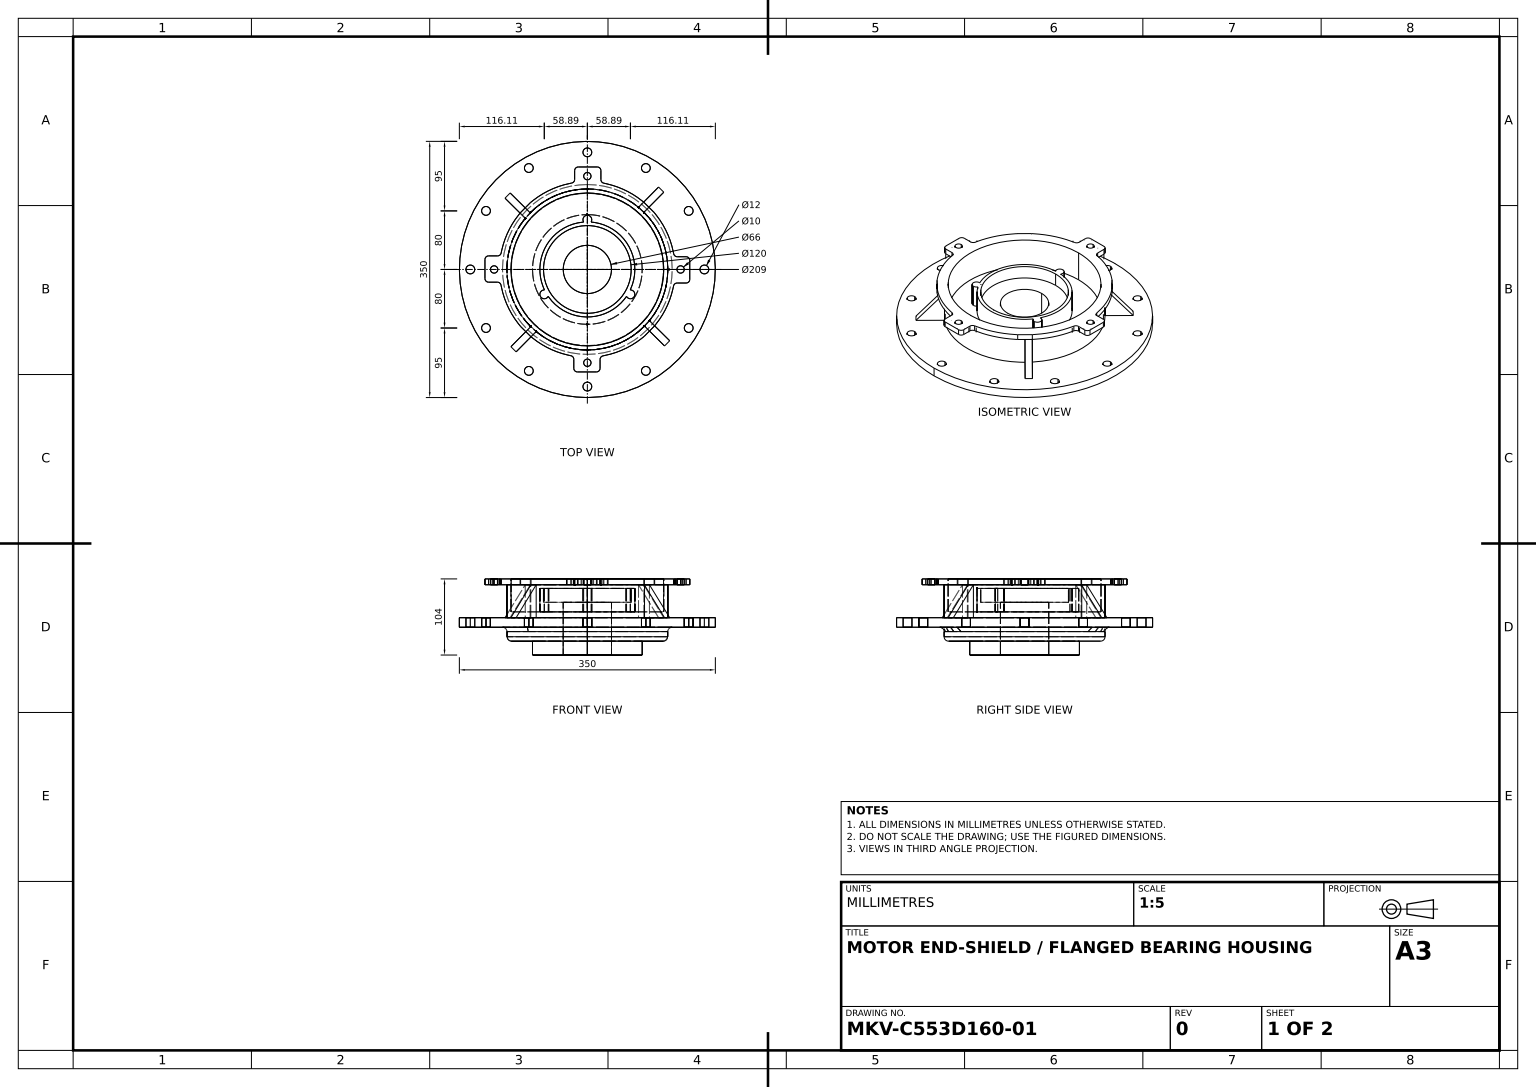
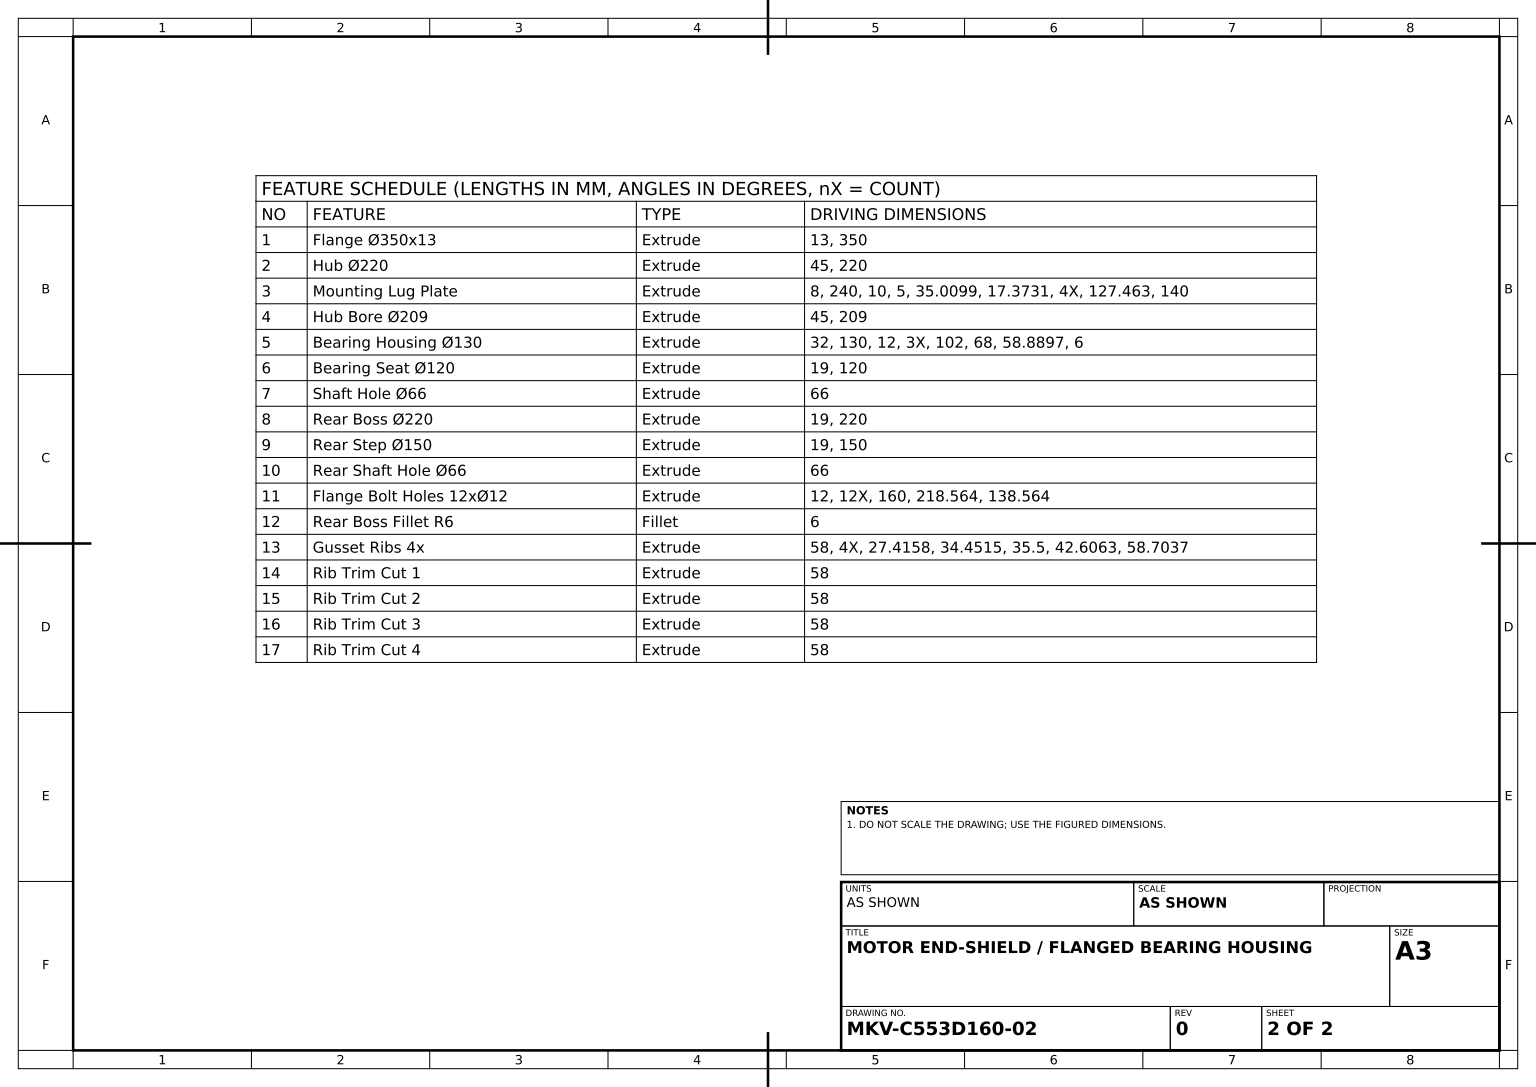
SolidWorks part; units mm, degrees
material "Plain Carbon Steel"
ref_plane "Front Plane" through (0, 0, 0) normal (0, 0, 1) x (1, 0, 0)
ref_plane "Top Plane" through (0, 0, 0) normal (0, 1, 0) x (1, 0, 0)
ref_plane "Right Plane" through (0, 0, 0) normal (1, 0, 0) x (0, 0, -1)
sketch "Flange Sketch" plane through (0, 0, 0) normal (0, 1, 0) x (1, 0, 0)
  circle A0 centre (0, 0) radius 175
  dimension "D1" = 350
extrude "Flange Ø350x13" add sketch "Flange Sketch" along normal blind 13
sketch "Hub Sketch" plane through (0, 13, 0) normal (0, 1, 0) x (1, 0, 0)
  circle A0 centre (0, 0) radius 110
  dimension "D1" = 220
extrude "Hub Ø220" add sketch "Hub Sketch" along normal blind 45
sketch "Lug Plate Sketch" plane through (0, 58, 0) normal (0, 1, 0) x (1, 0, 0)
  line L0 (122.9815, 17.3731) -> (135, 17.3731)
  line L2 (-17.3731, 122.9815) -> (-17.3731, 135)
  line L3 (-12.3731, 140) -> (13.5317, 140)
  line L4 (18.5317, 122.7651) -> (18.5317, 135)
  line L5 (140, 12.3731) -> (140, -13.5317)
  line L6 (122.7651, -18.5317) -> (135, -18.5317)
  line L7 (17.3731, -122.9815) -> (17.3731, -135)
  line L8 (12.3731, -140) -> (-13.5317, -140)
  line L9 (-18.5317, -122.7651) -> (-18.5317, -135)
  line L10 (-122.9815, -17.3731) -> (-135, -17.3731)
  line L11 (-140, -12.3731) -> (-140, 13.5317)
  line L12 (-122.7651, 18.5317) -> (-135, 18.5317)
  arc A0 (-21.4782, 118.0622) -> (-117.8545, 22.5904) centre (0, 0) ccw
  circle A2 centre (0, 127.4634) radius 5
  arc A3 (-17.3731, 122.9815) -> (-21.4782, 118.0622) centre (-22.3731, 122.9815) cw
  arc A4 (18.5317, 122.7651) -> (22.5904, 117.8545) centre (23.5317, 122.7651) ccw
  arc A5 (18.5317, 135) -> (13.5317, 140) centre (13.5317, 135) ccw
  arc A6 (-12.3731, 140) -> (-17.3731, 135) centre (-12.3731, 135) ccw
  arc A7 (122.9815, 17.3731) -> (118.0622, 21.4782) centre (122.9815, 22.3731) cw
  arc A8 (140, 12.3731) -> (135, 17.3731) centre (135, 12.3731) ccw
  arc A9 (135, -18.5317) -> (140, -13.5317) centre (135, -13.5317) ccw
  arc A10 (122.7651, -18.5317) -> (117.8545, -22.5904) centre (122.7651, -23.5317) ccw
  circle A11 centre (127.4634, 0) radius 5
  arc A12 (17.3731, -122.9815) -> (21.4782, -118.0622) centre (22.3731, -122.9815) cw
  arc A13 (12.3731, -140) -> (17.3731, -135) centre (12.3731, -135) ccw
  arc A14 (-18.5317, -135) -> (-13.5317, -140) centre (-13.5317, -135) ccw
  arc A15 (-18.5317, -122.7651) -> (-22.5904, -117.8545) centre (-23.5317, -122.7651) ccw
  circle A16 centre (0, -127.4634) radius 5
  arc A17 (-122.9815, -17.3731) -> (-118.0622, -21.4782) centre (-122.9815, -22.3731) cw
  arc A18 (-140, -12.3731) -> (-135, -17.3731) centre (-135, -12.3731) ccw
  arc A19 (-135, 18.5317) -> (-140, 13.5317) centre (-135, 13.5317) ccw
  arc A20 (-122.7651, 18.5317) -> (-117.8545, 22.5904) centre (-122.7651, 23.5317) ccw
  circle A21 centre (-127.4634, 0) radius 5
  arc A22 (-118.0622, -21.4782) -> (-22.5904, -117.8545) centre (0, 0) ccw
  arc A23 (118.0622, 21.4782) -> (22.5904, 117.8545) centre (0, 0) ccw
  arc A24 (21.4782, -118.0622) -> (117.8545, -22.5904) centre (0, 0) ccw
  point P16 (18.5317, 140)
  dimension "D1" = 240
  dimension "D2" = 127.4634
  dimension "D3" = 10
  dimension "D5" = 5
  dimension "D6" = 5
  dimension "D7" = 5
  dimension "D11" = 4
  dimension "D8" = 35.0099
  dimension "D10" = 17.3731
  dimension "D12" = 127.4634
  dimension "D13" = 140
extrude "Mounting Lug Plate" add sketch "Lug Plate Sketch" along normal blind 8
sketch "Hub Bore Sketch" plane through (0, 66, 0) normal (0, 1, 0) x (1, 0, 0)
  circle A0 centre (0, 0) radius 104.5
  dimension "D1" = 209
extrude "Hub Bore Ø209" cut sketch "Hub Bore Sketch" against normal blind 45
sketch "Bearing Housing Sketch" plane through (0, 21, 0) normal (0, 1, 0) x (1, 0, 0)
  circle A0 centre (0, 0) radius 65
  arc A1 (5.0764, 64.8015) -> (-5.0764, 64.8015) centre (0, 68) ccw
  circle A2 centre (0, 68) radius 3
  arc A3 (53.5815, -36.797) -> (58.6579, -28.0045) centre (58.8897, -34) ccw
  circle A4 centre (58.8897, -34) radius 3
  arc A5 (-58.6579, -28.0045) -> (-53.5815, -36.797) centre (-58.8897, -34) ccw
  circle A6 centre (-58.8897, -34) radius 3
  dimension "D1" = 130
  dimension "D2" = 12
  dimension "D3" = 3
  dimension "D7" = 6
  dimension "D4" = 102
  dimension "D5" = 68
  dimension "D6" = 58.8897
  dimension "D8" = 58.8897
extrude "Bearing Housing Ø130" add sketch "Bearing Housing Sketch" along normal blind 32 contours A0 A2 A1 | A2 | A0 A6 A5 | A6 | A0 A4 A3 | A4 | A0
sketch "Bearing Seat Sketch" plane through (0, 53, 0) normal (0, 1, 0) x (1, 0, 0)
  circle A0 centre (0, 0) radius 60
  dimension "D1" = 120
extrude "Bearing Seat Ø120" cut sketch "Bearing Seat Sketch" against normal blind 19
sketch "Shaft Hole Sketch" plane through (0, 34, 0) normal (0, 1, 0) x (1, 0, 0)
  circle A0 centre (0, 0) radius 33
  dimension "D1" = 66
extrude "Shaft Hole Ø66" cut sketch "Shaft Hole Sketch" against normal through all
sketch "Rear Boss Sketch" plane through (0, 0, 0) normal (0, -1, 0) x (1, 0, 0)
  circle A0 centre (0, 0) radius 110
  dimension "D1" = 220
extrude "Rear Boss Ø220" add sketch "Rear Boss Sketch" along normal blind 19
sketch "Rear Step Sketch" plane through (0, -19, 0) normal (0, -1, 0) x (1, 0, 0)
  circle A0 centre (0, 0) radius 75
  dimension "D1" = 150
extrude "Rear Step Ø150" add sketch "Rear Step Sketch" along normal blind 19
sketch "Rear Shaft Hole Sketch" plane through (0, -38, 0) normal (0, -1, 0) x (1, 0, 0)
  circle A0 centre (0, 0) radius 33
  dimension "D1" = 66
extrude "Rear Shaft Hole Ø66" cut sketch "Rear Shaft Hole Sketch" against normal through all
sketch "Flange Bolt Holes Sketch" plane through (0, 13, 0) normal (0, 1, 0) x (1, 0, 0)
  circle A1 centre (0, 160) radius 6
  circle A2 centre (80, 138.5641) radius 6
  circle A3 centre (138.5641, 80) radius 6
  circle A4 centre (160, 0) radius 6
  circle A5 centre (138.5641, -80) radius 6
  circle A6 centre (80, -138.5641) radius 6
  circle A7 centre (0, -160) radius 6
  circle A8 centre (-80, -138.5641) radius 6
  circle A9 centre (-138.5641, -80) radius 6
  circle A10 centre (-160, 0) radius 6
  circle A11 centre (-138.5641, 80) radius 6
  circle A12 centre (-80, 138.5641) radius 6
  dimension "D1" = 160
  dimension "D2" = 12
  dimension "D6" = 138.5641
  dimension "D4" = 218.5641
  dimension "D5" = 218.5641
  dimension "D3" = 12
extrude "Flange Bolt Holes 12xØ12" cut sketch "Flange Bolt Holes Sketch" against normal through all
fillet "Rear Boss Fillet R6" radius 6 2 edges at (0, -19, -110) (0, 0, 110)
sketch "Gusset Ribs Sketch" plane through (0, 66, 0) normal (0, 1, 0) x (1, 0, 0)
  line L0 (-74.2606, 73.5229) -> (-105.5485, 104.5)
  line L1 (-74.2606, 73.5229) -> (-81.2963, 66.4166)
  line L2 (-105.5485, 104.5) -> (-112.5842, 97.3937)
  line L3 (-81.2963, 66.4166) -> (-112.5842, 97.3937)
  line L4 (104.5, 105.5485) -> (97.3937, 112.5842)
  line L5 (73.5229, 74.2606) -> (104.5, 105.5485)
  line L6 (66.4166, 81.2963) -> (97.3937, 112.5842)
  line L7 (105.5485, -104.5) -> (112.5842, -97.3937)
  line L8 (74.2606, -73.5229) -> (105.5485, -104.5)
  line L9 (81.2963, -66.4166) -> (112.5842, -97.3937)
  line L10 (-104.5, -105.5485) -> (-97.3937, -112.5842)
  line L11 (-73.5229, -74.2606) -> (-104.5, -105.5485)
  line L12 (-66.4166, -81.2963) -> (-97.3937, -112.5842)
  line L13 (66.4166, 81.2963) -> (73.5229, 74.2606)
  line L14 (81.2963, -66.4166) -> (74.2606, -73.5229)
  line L15 (-73.5229, -74.2606) -> (-66.4166, -81.2963)
  line L16 (-140, 13.5317) -> (-140, -12.3731) construction
  circle A0 centre (0, 0) radius 104.5 construction
  dimension "D1" = 4
  dimension "D2" = 27.4158
  dimension "D3" = 34.4515
  dimension "D4" = 35.5
  dimension "D5" = 42.6063
  dimension "D6" = 58.7037
extrude "Gusset Ribs 4x" add sketch "Gusset Ribs Sketch" against normal blind 58
sketch "Rib Trim Sketch 1" plane through (7.1063, 0, 7.0357) normal (0.7106, 0, 0.7036) x (0.7036, 0, -0.7106)
  line L0 (-109.5445, 58) -> (-148.5286, 13)
  line L1 (-148.5286, 13) -> (-148.5286, 66)
  line L2 (-148.5286, 66) -> (-119.5826, 66)
  line L3 (-119.5826, 66) -> (-119.5826, 58)
  line L4 (-119.5826, 58) -> (-109.5445, 58)
extrude "Rib Trim Cut 1" cut sketch "Rib Trim Sketch 1" against normal blind 58
sketch "Rib Trim Sketch 2" plane through (-7.0357, 0, 7.1063) normal (-0.7036, 0, 0.7106) x (0.7106, 0, 0.7036)
  line L0 (-109.5445, 58) -> (-148.5286, 13)
  line L1 (-148.5286, 13) -> (-148.5286, 66)
  line L2 (-148.5286, 66) -> (-119.5826, 66)
  line L3 (-148.5286, 66) -> (-119.5826, 66) construction
  line L4 (-119.5826, 66) -> (-119.5826, 58)
  line L5 (-119.5826, 58) -> (-109.5445, 58)
extrude "Rib Trim Cut 2" cut sketch "Rib Trim Sketch 2" against normal blind 58
sketch "Rib Trim Sketch 3" plane through (-7.1063, 0, -7.0357) normal (-0.7106, 0, -0.7036) x (-0.7036, 0, 0.7106)
  line L0 (-109.5445, 58) -> (-148.5286, 13)
  line L1 (-148.5286, 13) -> (-148.5286, 66)
  line L2 (-148.5286, 66) -> (-119.5826, 66)
  line L3 (-119.5826, 66) -> (-119.5826, 58)
  line L4 (-119.5826, 58) -> (-109.5445, 58)
extrude "Rib Trim Cut 3" cut sketch "Rib Trim Sketch 3" against normal blind 58
sketch "Rib Trim Sketch 4" plane through (7.0357, 0, -7.1063) normal (0.7036, 0, -0.7106) x (-0.7106, 0, -0.7036)
  line L0 (-109.5445, 58) -> (-148.5286, 13)
  line L1 (-148.5286, 13) -> (-148.5286, 66)
  line L2 (-148.5286, 66) -> (-119.5826, 66)
  line L3 (-119.5826, 66) -> (-119.5826, 58)
  line L4 (-119.5826, 58) -> (-109.5445, 58)
extrude "Rib Trim Cut 4" cut sketch "Rib Trim Sketch 4" against normal blind 58
